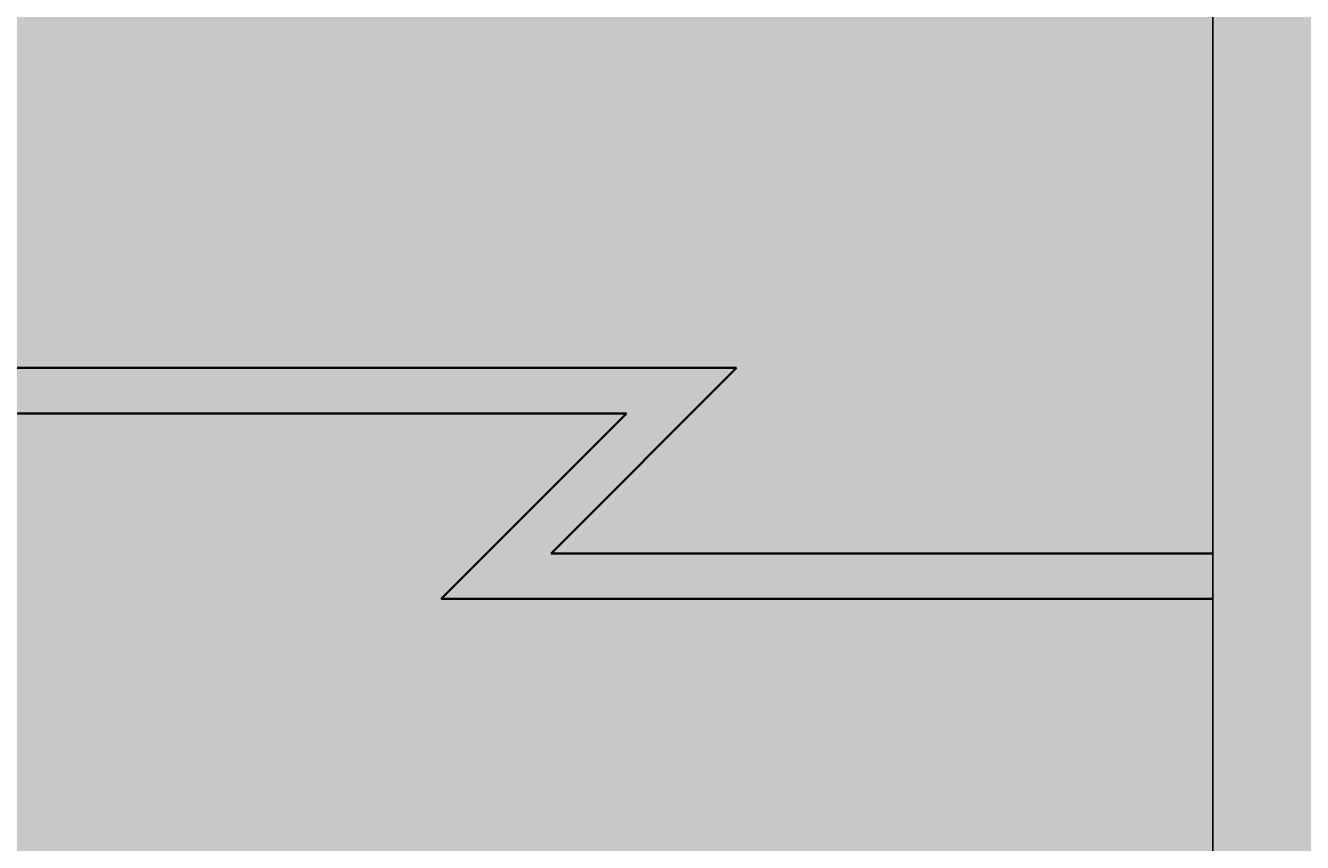
# Model space of a CAD drawing. Units: millimetres. Extents: x -22994 to 29398, y -19990 to 20176.
# Tile 47 of 135: x 170 to 198, y 78 to 96. Entities that reach past the tile are written whole.
import ezdxf
from ezdxf import colors
from ezdxf.entities.mleader import LeaderData, LeaderLine
from ezdxf.math import Vec2, Vec3

# ---------------------------------------------------------------- set-up
doc = ezdxf.new("R2010")
doc.units = ezdxf.units.MM
doc.header["$MEASUREMENT"] = 0
for name, color, linetype, lineweight in [('M-ANNO-TEXT', 7, 'Continuous', 25), ('M-DIMS', 2, 'Continuous', 18), ('M-EQPM', 7, 'Continuous', 25), ('M-EQPM-PATT', 7, 'Continuous', 18), ('M-PIPE', 7, 'Continuous', 35)]:
    doc.layers.add(name, color=color, linetype=linetype, lineweight=lineweight)
doc.styles.get("Standard").update_dxf_attribs({"font": 'arial.ttf'})
doc.dimstyles.get("Standard").update_dxf_attribs({"dimtxt": 0.18, "dimasz": 10000, "dimexe": 0.18, "dimexo": 0.0625, "dimgap": 0.09, "dimtad": 0, "dimtih": 1, "dimtoh": 1, "dimdec": 0, "dimzin": 0, "dimdsep": 46, "dimtxsty": 'Standard', "dimcen": 0.09, "dimadec": 0, "dimazin": 0, "dimtfac": 1, "dimtdec": 0, "dimtofl": 0, "dimtmove": 0, "dimatfit": 3, "dimfxl": 1, "dimtolj": 1, "dimtzin": 0, "dimlwd": 30, "dimarcsym": 0})

# ---------------------------------------------------------------- blocks, each defined once
blk = doc.blocks.new('*D2')
at = {"layer": 'Defpoints', "color": 0, "transparency": 16777216}
for p in [(6.677, 10.271), (290.852, 10.271), (290.852, -5.079)]:
    blk.add_point(p, dxfattribs=at)
at = {"layer": 'M-DIMS', "color": 0, "lineweight": -2, "transparency": 16777216}
for p, q in [((6.677, 10.209), (6.677, -5.259)), ((290.852, 10.209), (290.852, -5.259))]:
    blk.add_line(p, q, dxfattribs=at)
at = {"layer": 'M-DIMS', "color": 0, "lineweight": 30, "transparency": 16777216}
for p, q in [((-9993.323, -5.079), (-19993.323, -5.079)), ((10290.852, -5.079), (20290.852, -5.079))]:
    blk.add_line(p, q, dxfattribs=at)
at = {"layer": 'M-DIMS', "color": 0, "transparency": 16777216}
for points in [[(-9993.323, 1661.588), (-9993.323, -1671.745), (6.677, -5.079)], [(10290.852, 1661.588), (10290.852, -1671.745), (290.852, -5.079)]]:
    blk.add_solid(points, dxfattribs=at)
at = {"layer": 'M-DIMS', "color": 0, "transparency": 16777216, "insert": (148.765, -5.079), "char_height": 0.18, "attachment_point": 5}
blk.add_mtext('\\A1;284.2', dxfattribs=at)
blk = doc.blocks.new('*D3')
at = {"layer": 'Defpoints', "color": 0, "transparency": 16777216}
for p in [(110.265, 204.165), (110.265, 176.366), (95.833, 127.967)]:
    blk.add_point(p, dxfattribs=at)
at = {"layer": 'M-DIMS', "color": 0, "lineweight": 30, "transparency": 16777216}
for p, q in [((-9904.167, 204.165), (-19904.167, 204.165)), ((10110.265, 204.165), (20110.265, 204.165))]:
    blk.add_line(p, q, dxfattribs=at)
at = {"layer": 'M-DIMS', "color": 0, "lineweight": -2, "transparency": 16777216}
for p, q in [((95.833, 128.03), (95.833, 204.345)), ((110.265, 176.429), (110.265, 204.345))]:
    blk.add_line(p, q, dxfattribs=at)
at = {"layer": 'M-DIMS', "color": 0, "transparency": 16777216}
for points in [[(-9904.167, 1870.832), (-9904.167, -1462.501), (95.833, 204.165)], [(10110.265, 1870.832), (10110.265, -1462.501), (110.265, 204.165)]]:
    blk.add_solid(points, dxfattribs=at)
at = {"layer": 'M-DIMS', "color": 0, "transparency": 16777216, "insert": (103.049, 204.165), "char_height": 0.18, "attachment_point": 5}
blk.add_mtext('\\A1;14.432', dxfattribs=at)
blk = doc.blocks.new('*D4')
at = {"layer": 'Defpoints', "color": 0, "transparency": 16777216}
for p in [(116.265, 204.165), (110.265, 176.366), (116.265, 176.366)]:
    blk.add_point(p, dxfattribs=at)
at = {"layer": 'M-DIMS', "color": 0, "lineweight": 30, "transparency": 16777216}
for p, q in [((-9889.735, 204.165), (-19889.735, 204.165)), ((10116.265, 204.165), (20116.265, 204.165))]:
    blk.add_line(p, q, dxfattribs=at)
at = {"layer": 'M-DIMS', "color": 0, "lineweight": -2, "transparency": 16777216}
for p, q in [((110.265, 176.429), (110.265, 204.345)), ((116.265, 176.429), (116.265, 204.345))]:
    blk.add_line(p, q, dxfattribs=at)
at = {"layer": 'M-DIMS', "color": 0, "transparency": 16777216}
for points in [[(-9889.735, 1870.832), (-9889.735, -1462.501), (110.265, 204.165)], [(10116.265, 1870.832), (10116.265, -1462.501), (116.265, 204.165)]]:
    blk.add_solid(points, dxfattribs=at)
at = {"layer": 'M-DIMS', "color": 0, "transparency": 16777216, "insert": (113.265, 204.165), "char_height": 0.18, "attachment_point": 5}
blk.add_mtext('\\A1;6', dxfattribs=at)
blk = doc.blocks.new('*D5')
at = {"layer": 'Defpoints', "color": 0, "transparency": 16777216}
for p in [(181.265, 204.165), (116.265, 176.366), (181.265, 176.366)]:
    blk.add_point(p, dxfattribs=at)
at = {"layer": 'M-DIMS', "color": 0, "lineweight": 30, "transparency": 16777216}
for p, q in [((-9883.735, 204.165), (-19883.735, 204.165)), ((10181.265, 204.165), (20181.265, 204.165))]:
    blk.add_line(p, q, dxfattribs=at)
at = {"layer": 'M-DIMS', "color": 0, "lineweight": -2, "transparency": 16777216}
for p, q in [((116.265, 176.429), (116.265, 204.345)), ((181.265, 176.429), (181.265, 204.345))]:
    blk.add_line(p, q, dxfattribs=at)
at = {"layer": 'M-DIMS', "color": 0, "transparency": 16777216}
for points in [[(-9883.735, 1870.832), (-9883.735, -1462.501), (116.265, 204.165)], [(10181.265, 1870.832), (10181.265, -1462.501), (181.265, 204.165)]]:
    blk.add_solid(points, dxfattribs=at)
at = {"layer": 'M-DIMS', "color": 0, "transparency": 16777216, "insert": (148.765, 204.165), "char_height": 0.18, "attachment_point": 5}
blk.add_mtext('\\A1;65', dxfattribs=at)
blk = doc.blocks.new('*D6')
at = {"layer": 'Defpoints', "color": 0, "transparency": 16777216}
for p in [(187.265, 204.165), (181.265, 176.366), (187.265, 176.366)]:
    blk.add_point(p, dxfattribs=at)
at = {"layer": 'M-DIMS', "color": 0, "lineweight": 30, "transparency": 16777216}
for p, q in [((-9818.735, 204.165), (-19818.735, 204.165)), ((10187.265, 204.165), (20187.265, 204.165))]:
    blk.add_line(p, q, dxfattribs=at)
at = {"layer": 'M-DIMS', "color": 0, "lineweight": -2, "transparency": 16777216}
for p, q in [((181.265, 176.429), (181.265, 204.345)), ((187.265, 176.429), (187.265, 204.345))]:
    blk.add_line(p, q, dxfattribs=at)
at = {"layer": 'M-DIMS', "color": 0, "transparency": 16777216}
for points in [[(-9818.735, 1870.832), (-9818.735, -1462.501), (181.265, 204.165)], [(10187.265, 1870.832), (10187.265, -1462.501), (187.265, 204.165)]]:
    blk.add_solid(points, dxfattribs=at)
at = {"layer": 'M-DIMS', "color": 0, "transparency": 16777216, "insert": (184.265, 204.165), "char_height": 0.18, "attachment_point": 5}
blk.add_mtext('\\A1;6', dxfattribs=at)
blk = doc.blocks.new('*D7')
at = {"layer": 'Defpoints', "color": 0, "transparency": 16777216}
for p in [(201.697, 204.165), (187.265, 176.366), (201.697, 127.967)]:
    blk.add_point(p, dxfattribs=at)
at = {"layer": 'M-DIMS', "color": 0, "lineweight": 30, "transparency": 16777216}
for p, q in [((-9812.735, 204.165), (-19812.735, 204.165)), ((10201.697, 204.165), (20201.697, 204.165))]:
    blk.add_line(p, q, dxfattribs=at)
at = {"layer": 'M-DIMS', "color": 0, "lineweight": -2, "transparency": 16777216}
for p, q in [((187.265, 176.429), (187.265, 204.345)), ((201.697, 128.03), (201.697, 204.345))]:
    blk.add_line(p, q, dxfattribs=at)
at = {"layer": 'M-DIMS', "color": 0, "transparency": 16777216}
for points in [[(-9812.735, 1870.832), (-9812.735, -1462.501), (187.265, 204.165)], [(10201.697, 1870.832), (10201.697, -1462.501), (201.697, 204.165)]]:
    blk.add_solid(points, dxfattribs=at)
at = {"layer": 'M-DIMS', "color": 0, "transparency": 16777216, "insert": (194.481, 204.165), "char_height": 0.18, "attachment_point": 5}
blk.add_mtext('\\A1;14.432', dxfattribs=at)
blk = doc.blocks.new('*D8')
at = {"layer": 'Defpoints', "color": 0, "transparency": 16777216}
for p in [(227.648, 204.165), (227.648, 146.73), (201.697, 127.967)]:
    blk.add_point(p, dxfattribs=at)
at = {"layer": 'M-DIMS', "color": 0, "lineweight": 30, "transparency": 16777216}
for p, q in [((-9798.303, 204.165), (-19798.303, 204.165)), ((10227.648, 204.165), (20227.648, 204.165))]:
    blk.add_line(p, q, dxfattribs=at)
at = {"layer": 'M-DIMS', "color": 0, "lineweight": -2, "transparency": 16777216}
for p, q in [((201.697, 128.03), (201.697, 204.345)), ((227.648, 146.792), (227.648, 204.345))]:
    blk.add_line(p, q, dxfattribs=at)
at = {"layer": 'M-DIMS', "color": 0, "transparency": 16777216}
for points in [[(-9798.303, 1870.832), (-9798.303, -1462.501), (201.697, 204.165)], [(10227.648, 1870.832), (10227.648, -1462.501), (227.648, 204.165)]]:
    blk.add_solid(points, dxfattribs=at)
at = {"layer": 'M-DIMS', "color": 0, "transparency": 16777216, "insert": (214.673, 204.165), "char_height": 0.18, "attachment_point": 5}
blk.add_mtext('\\A1;25.95', dxfattribs=at)
blk = doc.blocks.new('*D9')
at = {"layer": 'Defpoints', "color": 0, "transparency": 16777216}
for p in [(187.265, 176.366), (306.202, 176.366), (290.852, 10.271)]:
    blk.add_point(p, dxfattribs=at)
at = {"layer": 'M-DIMS', "color": 0, "lineweight": 30, "transparency": 16777216}
for p, q in [((306.202, 10176.366), (306.202, 20176.366)), ((306.202, -9989.729), (306.202, -19989.729))]:
    blk.add_line(p, q, dxfattribs=at)
at = {"layer": 'M-DIMS', "color": 0, "lineweight": -2, "transparency": 16777216}
for p, q in [((187.327, 176.366), (306.382, 176.366)), ((290.915, 10.271), (306.382, 10.271))]:
    blk.add_line(p, q, dxfattribs=at)
at = {"layer": 'M-DIMS', "color": 0, "transparency": 16777216}
for points in [[(-1360.465, 10176.366), (1972.869, 10176.366), (306.202, 176.366)], [(-1360.465, -9989.729), (1972.869, -9989.729), (306.202, 10.271)]]:
    blk.add_solid(points, dxfattribs=at)
at = {"layer": 'M-DIMS', "color": 0, "transparency": 16777216, "insert": (306.202, 93.319), "char_height": 0.18, "attachment_point": 5}
blk.add_mtext('\\A1;166.1', dxfattribs=at)
blk = doc.blocks.new('*D10')
at = {"layer": 'Defpoints', "color": 0, "transparency": 16777216}
for p in [(125.65, 136.071), (133.346, 136.071), (133.346, -5.079)]:
    blk.add_point(p, dxfattribs=at)
at = {"layer": 'M-DIMS', "color": 0, "lineweight": -2, "transparency": 16777216}
for p, q in [((125.65, 136.009), (125.65, -5.259)), ((133.346, 136.009), (133.346, -5.259))]:
    blk.add_line(p, q, dxfattribs=at)
at = {"layer": 'M-DIMS', "color": 0, "lineweight": 30, "transparency": 16777216}
for p, q in [((-9874.35, -5.079), (-19874.35, -5.079)), ((10133.346, -5.079), (20133.346, -5.079))]:
    blk.add_line(p, q, dxfattribs=at)
at = {"layer": 'M-DIMS', "color": 0, "transparency": 16777216}
for points in [[(-9874.35, 1661.588), (-9874.35, -1671.745), (125.65, -5.079)], [(10133.346, 1661.588), (10133.346, -1671.745), (133.346, -5.079)]]:
    blk.add_solid(points, dxfattribs=at)
at = {"layer": 'M-DIMS', "color": 0, "transparency": 16777216, "insert": (129.498, -5.079), "char_height": 0.18, "attachment_point": 5}
blk.add_mtext('\\A1;7.696', dxfattribs=at)
blk = doc.blocks.new('*D11')
at = {"layer": 'Defpoints', "color": 0, "transparency": 16777216}
for p in [(133.346, 136.071), (135.65, 136.071), (135.65, -5.079)]:
    blk.add_point(p, dxfattribs=at)
at = {"layer": 'M-DIMS', "color": 0, "lineweight": -2, "transparency": 16777216}
for p, q in [((133.346, 136.009), (133.346, -5.259)), ((135.65, 136.009), (135.65, -5.259))]:
    blk.add_line(p, q, dxfattribs=at)
at = {"layer": 'M-DIMS', "color": 0, "lineweight": 30, "transparency": 16777216}
for p, q in [((-9866.654, -5.079), (-19866.654, -5.079)), ((10135.65, -5.079), (20135.65, -5.079))]:
    blk.add_line(p, q, dxfattribs=at)
at = {"layer": 'M-DIMS', "color": 0, "transparency": 16777216}
for points in [[(-9866.654, 1661.588), (-9866.654, -1671.745), (133.346, -5.079)], [(10135.65, 1661.588), (10135.65, -1671.745), (135.65, -5.079)]]:
    blk.add_solid(points, dxfattribs=at)
at = {"layer": 'M-DIMS', "color": 0, "transparency": 16777216, "insert": (134.498, -5.079), "char_height": 0.18, "attachment_point": 5}
blk.add_mtext('\\A1;2.304', dxfattribs=at)
blk = doc.blocks.new('*D12')
at = {"layer": 'Defpoints', "color": 0, "transparency": 16777216}
for p in [(135.65, 136.071), (145.65, 136.071), (145.65, -5.079)]:
    blk.add_point(p, dxfattribs=at)
at = {"layer": 'M-DIMS', "color": 0, "lineweight": -2, "transparency": 16777216}
for p, q in [((135.65, 136.009), (135.65, -5.259)), ((145.65, 136.009), (145.65, -5.259))]:
    blk.add_line(p, q, dxfattribs=at)
at = {"layer": 'M-DIMS', "color": 0, "lineweight": 30, "transparency": 16777216}
for p, q in [((-9864.35, -5.079), (-19864.35, -5.079)), ((10145.65, -5.079), (20145.65, -5.079))]:
    blk.add_line(p, q, dxfattribs=at)
at = {"layer": 'M-DIMS', "color": 0, "transparency": 16777216}
for points in [[(-9864.35, 1661.588), (-9864.35, -1671.745), (135.65, -5.079)], [(10145.65, 1661.588), (10145.65, -1671.745), (145.65, -5.079)]]:
    blk.add_solid(points, dxfattribs=at)
at = {"layer": 'M-DIMS', "color": 0, "transparency": 16777216, "insert": (140.65, -5.079), "char_height": 0.18, "attachment_point": 5}
blk.add_mtext('\\A1;10', dxfattribs=at)
blk = doc.blocks.new('*D13')
at = {"layer": 'Defpoints', "color": 0, "transparency": 16777216}
for p in [(145.65, 136.071), (155.65, 136.071), (155.65, -5.079)]:
    blk.add_point(p, dxfattribs=at)
at = {"layer": 'M-DIMS', "color": 0, "lineweight": -2, "transparency": 16777216}
for p, q in [((145.65, 136.009), (145.65, -5.259)), ((155.65, 136.009), (155.65, -5.259))]:
    blk.add_line(p, q, dxfattribs=at)
at = {"layer": 'M-DIMS', "color": 0, "lineweight": 30, "transparency": 16777216}
for p, q in [((-9854.35, -5.079), (-19854.35, -5.079)), ((10155.65, -5.079), (20155.65, -5.079))]:
    blk.add_line(p, q, dxfattribs=at)
at = {"layer": 'M-DIMS', "color": 0, "transparency": 16777216}
for points in [[(-9854.35, 1661.588), (-9854.35, -1671.745), (145.65, -5.079)], [(10155.65, 1661.588), (10155.65, -1671.745), (155.65, -5.079)]]:
    blk.add_solid(points, dxfattribs=at)
at = {"layer": 'M-DIMS', "color": 0, "transparency": 16777216, "insert": (150.65, -5.079), "char_height": 0.18, "attachment_point": 5}
blk.add_mtext('\\A1;10', dxfattribs=at)
blk = doc.blocks.new('*D14')
at = {"layer": 'Defpoints', "color": 0, "transparency": 16777216}
for p in [(155.65, 136.071), (165.65, 136.071), (165.65, -5.079)]:
    blk.add_point(p, dxfattribs=at)
at = {"layer": 'M-DIMS', "color": 0, "lineweight": -2, "transparency": 16777216}
for p, q in [((155.65, 136.009), (155.65, -5.259)), ((165.65, 136.009), (165.65, -5.259))]:
    blk.add_line(p, q, dxfattribs=at)
at = {"layer": 'M-DIMS', "color": 0, "lineweight": 30, "transparency": 16777216}
for p, q in [((-9844.35, -5.079), (-19844.35, -5.079)), ((10165.65, -5.079), (20165.65, -5.079))]:
    blk.add_line(p, q, dxfattribs=at)
at = {"layer": 'M-DIMS', "color": 0, "transparency": 16777216}
for points in [[(-9844.35, 1661.588), (-9844.35, -1671.745), (155.65, -5.079)], [(10165.65, 1661.588), (10165.65, -1671.745), (165.65, -5.079)]]:
    blk.add_solid(points, dxfattribs=at)
at = {"layer": 'M-DIMS', "color": 0, "transparency": 16777216, "insert": (160.65, -5.079), "char_height": 0.18, "attachment_point": 5}
blk.add_mtext('\\A1;10', dxfattribs=at)
blk = doc.blocks.new('*D15')
at = {"layer": 'Defpoints', "color": 0, "transparency": 16777216}
for p in [(173.346, 154.788), (173.346, 136.071), (306.202, 136.071)]:
    blk.add_point(p, dxfattribs=at)
at = {"layer": 'M-DIMS', "color": 0, "lineweight": 30, "transparency": 16777216}
for p, q in [((306.202, 10154.788), (306.202, 20154.788)), ((306.202, -9863.929), (306.202, -19863.929))]:
    blk.add_line(p, q, dxfattribs=at)
at = {"layer": 'M-DIMS', "color": 0, "lineweight": -2, "transparency": 16777216}
for p, q in [((173.408, 154.788), (306.382, 154.788)), ((173.408, 136.071), (306.382, 136.071))]:
    blk.add_line(p, q, dxfattribs=at)
at = {"layer": 'M-DIMS', "color": 0, "transparency": 16777216}
for points in [[(-1360.465, 10154.788), (1972.869, 10154.788), (306.202, 154.788)], [(-1360.465, -9863.929), (1972.869, -9863.929), (306.202, 136.071)]]:
    blk.add_solid(points, dxfattribs=at)
at = {"layer": 'M-DIMS', "color": 0, "transparency": 16777216, "insert": (306.202, 145.43), "char_height": 0.18, "attachment_point": 5}
blk.add_mtext('\\A1;18.717', dxfattribs=at)
blk = doc.blocks.new('*D16')
at = {"layer": 'Defpoints', "color": 0, "transparency": 16777216}
for p in [(120.17, 204.165), (110.466, 48.035), (120.17, 48.035)]:
    blk.add_point(p, dxfattribs=at)
at = {"layer": 'M-DIMS', "color": 0, "lineweight": 30, "transparency": 16777216}
for p, q in [((-9889.534, 204.165), (-19889.534, 204.165)), ((10120.17, 204.165), (20120.17, 204.165))]:
    blk.add_line(p, q, dxfattribs=at)
at = {"layer": 'M-DIMS', "color": 0, "lineweight": -2, "transparency": 16777216}
for p, q in [((110.466, 48.097), (110.466, 204.345)), ((120.17, 48.097), (120.17, 204.345))]:
    blk.add_line(p, q, dxfattribs=at)
at = {"layer": 'M-DIMS', "color": 0, "transparency": 16777216}
for points in [[(-9889.534, 1870.832), (-9889.534, -1462.501), (110.466, 204.165)], [(10120.17, 1870.832), (10120.17, -1462.501), (120.17, 204.165)]]:
    blk.add_solid(points, dxfattribs=at)
at = {"layer": 'M-DIMS', "color": 0, "transparency": 16777216, "insert": (115.318, 204.165), "char_height": 0.18, "attachment_point": 5}
blk.add_mtext('\\A1;9.704', dxfattribs=at)
blk = doc.blocks.new('*D17')
at = {"layer": 'Defpoints', "color": 0, "transparency": 16777216}
for p in [(126.17, 204.165), (120.17, 48.035), (126.17, 48.035)]:
    blk.add_point(p, dxfattribs=at)
at = {"layer": 'M-DIMS', "color": 0, "lineweight": 30, "transparency": 16777216}
for p, q in [((-9879.83, 204.165), (-19879.83, 204.165)), ((10126.17, 204.165), (20126.17, 204.165))]:
    blk.add_line(p, q, dxfattribs=at)
at = {"layer": 'M-DIMS', "color": 0, "lineweight": -2, "transparency": 16777216}
for p, q in [((120.17, 48.097), (120.17, 204.345)), ((126.17, 48.097), (126.17, 204.345))]:
    blk.add_line(p, q, dxfattribs=at)
at = {"layer": 'M-DIMS', "color": 0, "transparency": 16777216}
for points in [[(-9879.83, 1870.832), (-9879.83, -1462.501), (120.17, 204.165)], [(10126.17, 1870.832), (10126.17, -1462.501), (126.17, 204.165)]]:
    blk.add_solid(points, dxfattribs=at)
at = {"layer": 'M-DIMS', "color": 0, "transparency": 16777216, "insert": (123.17, 204.165), "char_height": 0.18, "attachment_point": 5}
blk.add_mtext('\\A1;6', dxfattribs=at)
blk = doc.blocks.new('*D18')
at = {"layer": 'Defpoints', "color": 0, "transparency": 16777216}
for p in [(132.17, 204.165), (126.17, 48.035), (132.17, 48.035)]:
    blk.add_point(p, dxfattribs=at)
at = {"layer": 'M-DIMS', "color": 0, "lineweight": 30, "transparency": 16777216}
for p, q in [((-9873.83, 204.165), (-19873.83, 204.165)), ((10132.17, 204.165), (20132.17, 204.165))]:
    blk.add_line(p, q, dxfattribs=at)
at = {"layer": 'M-DIMS', "color": 0, "lineweight": -2, "transparency": 16777216}
for p, q in [((126.17, 48.097), (126.17, 204.345)), ((132.17, 48.097), (132.17, 204.345))]:
    blk.add_line(p, q, dxfattribs=at)
at = {"layer": 'M-DIMS', "color": 0, "transparency": 16777216}
for points in [[(-9873.83, 1870.832), (-9873.83, -1462.501), (126.17, 204.165)], [(10132.17, 1870.832), (10132.17, -1462.501), (132.17, 204.165)]]:
    blk.add_solid(points, dxfattribs=at)
at = {"layer": 'M-DIMS', "color": 0, "transparency": 16777216, "insert": (129.17, 204.165), "char_height": 0.18, "attachment_point": 5}
blk.add_mtext('\\A1;6', dxfattribs=at)
blk = doc.blocks.new('*D19')
at = {"layer": 'Defpoints', "color": 0, "transparency": 16777216}
for p in [(138.17, 204.165), (132.17, 48.035), (138.17, 48.035)]:
    blk.add_point(p, dxfattribs=at)
at = {"layer": 'M-DIMS', "color": 0, "lineweight": 30, "transparency": 16777216}
for p, q in [((-9867.83, 204.165), (-19867.83, 204.165)), ((10138.17, 204.165), (20138.17, 204.165))]:
    blk.add_line(p, q, dxfattribs=at)
at = {"layer": 'M-DIMS', "color": 0, "lineweight": -2, "transparency": 16777216}
for p, q in [((132.17, 48.097), (132.17, 204.345)), ((138.17, 48.097), (138.17, 204.345))]:
    blk.add_line(p, q, dxfattribs=at)
at = {"layer": 'M-DIMS', "color": 0, "transparency": 16777216}
for points in [[(-9867.83, 1870.832), (-9867.83, -1462.501), (132.17, 204.165)], [(10138.17, 1870.832), (10138.17, -1462.501), (138.17, 204.165)]]:
    blk.add_solid(points, dxfattribs=at)
at = {"layer": 'M-DIMS', "color": 0, "transparency": 16777216, "insert": (135.17, 204.165), "char_height": 0.18, "attachment_point": 5}
blk.add_mtext('\\A1;6', dxfattribs=at)
blk = doc.blocks.new('*D20')
at = {"layer": 'Defpoints', "color": 0, "transparency": 16777216}
for p in [(144.17, 204.165), (138.17, 48.035), (144.17, 48.035)]:
    blk.add_point(p, dxfattribs=at)
at = {"layer": 'M-DIMS', "color": 0, "lineweight": 30, "transparency": 16777216}
for p, q in [((-9861.83, 204.165), (-19861.83, 204.165)), ((10144.17, 204.165), (20144.17, 204.165))]:
    blk.add_line(p, q, dxfattribs=at)
at = {"layer": 'M-DIMS', "color": 0, "lineweight": -2, "transparency": 16777216}
for p, q in [((138.17, 48.097), (138.17, 204.345)), ((144.17, 48.097), (144.17, 204.345))]:
    blk.add_line(p, q, dxfattribs=at)
at = {"layer": 'M-DIMS', "color": 0, "transparency": 16777216}
for points in [[(-9861.83, 1870.832), (-9861.83, -1462.501), (138.17, 204.165)], [(10144.17, 1870.832), (10144.17, -1462.501), (144.17, 204.165)]]:
    blk.add_solid(points, dxfattribs=at)
at = {"layer": 'M-DIMS', "color": 0, "transparency": 16777216, "insert": (141.17, 204.165), "char_height": 0.18, "attachment_point": 5}
blk.add_mtext('\\A1;6', dxfattribs=at)
blk = doc.blocks.new('*D21')
at = {"layer": 'Defpoints', "color": 0, "transparency": 16777216}
for p in [(149.116, 204.165), (144.17, 48.035), (149.116, 48.035)]:
    blk.add_point(p, dxfattribs=at)
at = {"layer": 'M-DIMS', "color": 0, "lineweight": 30, "transparency": 16777216}
for p, q in [((-9855.83, 204.165), (-19855.83, 204.165)), ((10149.116, 204.165), (20149.116, 204.165))]:
    blk.add_line(p, q, dxfattribs=at)
at = {"layer": 'M-DIMS', "color": 0, "lineweight": -2, "transparency": 16777216}
for p, q in [((144.17, 48.097), (144.17, 204.345)), ((149.116, 48.097), (149.116, 204.345))]:
    blk.add_line(p, q, dxfattribs=at)
at = {"layer": 'M-DIMS', "color": 0, "transparency": 16777216}
for points in [[(-9855.83, 1870.832), (-9855.83, -1462.501), (144.17, 204.165)], [(10149.116, 1870.832), (10149.116, -1462.501), (149.116, 204.165)]]:
    blk.add_solid(points, dxfattribs=at)
at = {"layer": 'M-DIMS', "color": 0, "transparency": 16777216, "insert": (146.643, 204.165), "char_height": 0.18, "attachment_point": 5}
blk.add_mtext('\\A1;4.945', dxfattribs=at)
blk = doc.blocks.new('*D22')
at = {"layer": 'Defpoints', "color": 0, "transparency": 16777216}
for p in [(149.116, 30.99), (155.116, 30.99), (155.116, -5.079)]:
    blk.add_point(p, dxfattribs=at)
at = {"layer": 'M-DIMS', "color": 0, "lineweight": -2, "transparency": 16777216}
for p, q in [((149.116, 30.927), (149.116, -5.259)), ((155.116, 30.927), (155.116, -5.259))]:
    blk.add_line(p, q, dxfattribs=at)
at = {"layer": 'M-DIMS', "color": 0, "lineweight": 30, "transparency": 16777216}
for p, q in [((-9850.884, -5.079), (-19850.884, -5.079)), ((10155.116, -5.079), (20155.116, -5.079))]:
    blk.add_line(p, q, dxfattribs=at)
at = {"layer": 'M-DIMS', "color": 0, "transparency": 16777216}
for points in [[(-9850.884, 1661.588), (-9850.884, -1671.745), (149.116, -5.079)], [(10155.116, 1661.588), (10155.116, -1671.745), (155.116, -5.079)]]:
    blk.add_solid(points, dxfattribs=at)
at = {"layer": 'M-DIMS', "color": 0, "transparency": 16777216, "insert": (152.116, -5.079), "char_height": 0.18, "attachment_point": 5}
blk.add_mtext('\\A1;6', dxfattribs=at)
blk = doc.blocks.new('*D23')
at = {"layer": 'Defpoints', "color": 0, "transparency": 16777216}
for p in [(155.116, 30.99), (161.116, 30.99), (161.116, -5.079)]:
    blk.add_point(p, dxfattribs=at)
at = {"layer": 'M-DIMS', "color": 0, "lineweight": -2, "transparency": 16777216}
for p, q in [((155.116, 30.927), (155.116, -5.259)), ((161.116, 30.927), (161.116, -5.259))]:
    blk.add_line(p, q, dxfattribs=at)
at = {"layer": 'M-DIMS', "color": 0, "lineweight": 30, "transparency": 16777216}
for p, q in [((-9844.884, -5.079), (-19844.884, -5.079)), ((10161.116, -5.079), (20161.116, -5.079))]:
    blk.add_line(p, q, dxfattribs=at)
at = {"layer": 'M-DIMS', "color": 0, "transparency": 16777216}
for points in [[(-9844.884, 1661.588), (-9844.884, -1671.745), (155.116, -5.079)], [(10161.116, 1661.588), (10161.116, -1671.745), (161.116, -5.079)]]:
    blk.add_solid(points, dxfattribs=at)
at = {"layer": 'M-DIMS', "color": 0, "transparency": 16777216, "insert": (158.116, -5.079), "char_height": 0.18, "attachment_point": 5}
blk.add_mtext('\\A1;6', dxfattribs=at)
blk = doc.blocks.new('*D24')
at = {"layer": 'Defpoints', "color": 0, "transparency": 16777216}
for p in [(161.116, 30.99), (166.439, 30.99), (166.439, -5.079)]:
    blk.add_point(p, dxfattribs=at)
at = {"layer": 'M-DIMS', "color": 0, "lineweight": -2, "transparency": 16777216}
for p, q in [((161.116, 30.927), (161.116, -5.259)), ((166.439, 30.927), (166.439, -5.259))]:
    blk.add_line(p, q, dxfattribs=at)
at = {"layer": 'M-DIMS', "color": 0, "lineweight": 30, "transparency": 16777216}
for p, q in [((-9838.884, -5.079), (-19838.884, -5.079)), ((10166.439, -5.079), (20166.439, -5.079))]:
    blk.add_line(p, q, dxfattribs=at)
at = {"layer": 'M-DIMS', "color": 0, "transparency": 16777216}
for points in [[(-9838.884, 1661.588), (-9838.884, -1671.745), (161.116, -5.079)], [(10166.439, 1661.588), (10166.439, -1671.745), (166.439, -5.079)]]:
    blk.add_solid(points, dxfattribs=at)
at = {"layer": 'M-DIMS', "color": 0, "transparency": 16777216, "insert": (163.777, -5.079), "char_height": 0.18, "attachment_point": 5}
blk.add_mtext('\\A1;5.323', dxfattribs=at)
blk = doc.blocks.new('*D25')
at = {"layer": 'Defpoints', "color": 0, "transparency": 16777216}
for p in [(166.439, 30.99), (172.439, 30.99), (172.439, -5.079)]:
    blk.add_point(p, dxfattribs=at)
at = {"layer": 'M-DIMS', "color": 0, "lineweight": -2, "transparency": 16777216}
for p, q in [((166.439, 30.927), (166.439, -5.259)), ((172.439, 30.927), (172.439, -5.259))]:
    blk.add_line(p, q, dxfattribs=at)
at = {"layer": 'M-DIMS', "color": 0, "lineweight": 30, "transparency": 16777216}
for p, q in [((-9833.561, -5.079), (-19833.561, -5.079)), ((10172.439, -5.079), (20172.439, -5.079))]:
    blk.add_line(p, q, dxfattribs=at)
at = {"layer": 'M-DIMS', "color": 0, "transparency": 16777216}
for points in [[(-9833.561, 1661.588), (-9833.561, -1671.745), (166.439, -5.079)], [(10172.439, 1661.588), (10172.439, -1671.745), (172.439, -5.079)]]:
    blk.add_solid(points, dxfattribs=at)
at = {"layer": 'M-DIMS', "color": 0, "transparency": 16777216, "insert": (169.439, -5.079), "char_height": 0.18, "attachment_point": 5}
blk.add_mtext('\\A1;6', dxfattribs=at)
blk = doc.blocks.new('*D26')
at = {"layer": 'Defpoints', "color": 0, "transparency": 16777216}
for p in [(172.439, 30.99), (178.439, 30.99), (178.439, -5.079)]:
    blk.add_point(p, dxfattribs=at)
at = {"layer": 'M-DIMS', "color": 0, "lineweight": -2, "transparency": 16777216}
for p, q in [((172.439, 30.927), (172.439, -5.259)), ((178.439, 30.927), (178.439, -5.259))]:
    blk.add_line(p, q, dxfattribs=at)
at = {"layer": 'M-DIMS', "color": 0, "lineweight": 30, "transparency": 16777216}
for p, q in [((-9827.561, -5.079), (-19827.561, -5.079)), ((10178.439, -5.079), (20178.439, -5.079))]:
    blk.add_line(p, q, dxfattribs=at)
at = {"layer": 'M-DIMS', "color": 0, "transparency": 16777216}
for points in [[(-9827.561, 1661.588), (-9827.561, -1671.745), (172.439, -5.079)], [(10178.439, 1661.588), (10178.439, -1671.745), (178.439, -5.079)]]:
    blk.add_solid(points, dxfattribs=at)
at = {"layer": 'M-DIMS', "color": 0, "transparency": 16777216, "insert": (175.439, -5.079), "char_height": 0.18, "attachment_point": 5}
blk.add_mtext('\\A1;6', dxfattribs=at)
blk = doc.blocks.new('*D27')
at = {"layer": 'Defpoints', "color": 0, "transparency": 16777216}
for p in [(178.439, 30.99), (188.117, 30.99), (188.117, -5.079)]:
    blk.add_point(p, dxfattribs=at)
at = {"layer": 'M-DIMS', "color": 0, "lineweight": -2, "transparency": 16777216}
for p, q in [((178.439, 30.927), (178.439, -5.259)), ((188.117, 30.927), (188.117, -5.259))]:
    blk.add_line(p, q, dxfattribs=at)
at = {"layer": 'M-DIMS', "color": 0, "lineweight": 30, "transparency": 16777216}
for p, q in [((-9821.561, -5.079), (-19821.561, -5.079)), ((10188.117, -5.079), (20188.117, -5.079))]:
    blk.add_line(p, q, dxfattribs=at)
at = {"layer": 'M-DIMS', "color": 0, "transparency": 16777216}
for points in [[(-9821.561, 1661.588), (-9821.561, -1671.745), (178.439, -5.079)], [(10188.117, 1661.588), (10188.117, -1671.745), (188.117, -5.079)]]:
    blk.add_solid(points, dxfattribs=at)
at = {"layer": 'M-DIMS', "color": 0, "transparency": 16777216, "insert": (183.278, -5.079), "char_height": 0.18, "attachment_point": 5}
blk.add_mtext('\\A1;9.679', dxfattribs=at)
blk = doc.blocks.new('*D28')
at = {"layer": 'Defpoints', "color": 0, "transparency": 16777216}
for p in [(188.117, 48.035), (306.202, 48.035), (188.117, 30.99)]:
    blk.add_point(p, dxfattribs=at)
at = {"layer": 'M-DIMS', "color": 0, "lineweight": 30, "transparency": 16777216}
for p, q in [((306.202, 10048.035), (306.202, 20048.035)), ((306.202, -9969.01), (306.202, -19969.01))]:
    blk.add_line(p, q, dxfattribs=at)
at = {"layer": 'M-DIMS', "color": 0, "lineweight": -2, "transparency": 16777216}
for p, q in [((188.18, 48.035), (306.382, 48.035)), ((188.18, 30.99), (306.382, 30.99))]:
    blk.add_line(p, q, dxfattribs=at)
at = {"layer": 'M-DIMS', "color": 0, "transparency": 16777216}
for points in [[(-1360.465, 10048.035), (1972.869, 10048.035), (306.202, 48.035)], [(-1360.465, -9969.01), (1972.869, -9969.01), (306.202, 30.99)]]:
    blk.add_solid(points, dxfattribs=at)
at = {"layer": 'M-DIMS', "color": 0, "transparency": 16777216, "insert": (306.202, 39.512), "char_height": 0.18, "attachment_point": 5}
blk.add_mtext('\\A1;17.045', dxfattribs=at)
blk = doc.blocks.new('*D29')
at = {"layer": 'Defpoints', "color": 0, "transparency": 16777216}
for p in [(36.801, 80.045), (64.03, 80.045)]:
    blk.add_point(p, dxfattribs=at)
at = {"layer": 'M-DIMS', "color": 0, "lineweight": -2, "transparency": 16777216}
for p, q in [((50.325, 80.045), (50.505, 80.045)), ((50.415, 79.955), (50.415, 80.135))]:
    blk.add_line(p, q, dxfattribs=at)
at = {"layer": 'M-DIMS', "color": 0, "lineweight": 30, "transparency": 16777216}
blk.add_line((20064.03, 80.03), (10064.03, 80.038), dxfattribs=at)
at = {"layer": 'M-DIMS', "color": 0, "transparency": 16777216}
blk.add_solid([(10064.031, 1746.704), (10064.028, -1586.629), (64.03, 80.045)], dxfattribs=at)
at = {"layer": 'M-DIMS', "color": 0, "transparency": 16777216, "insert": (20064.521, 80.03), "char_height": 0.18, "attachment_point": 5}
blk.add_mtext('\\A1;∅27.23', dxfattribs=at)
blk = doc.blocks.new('*D36')
at = {"layer": 'Defpoints', "color": 0, "transparency": 16777216}
for p in [(46.39, 31.303), (46.387, 26.593)]:
    blk.add_point(p, dxfattribs=at)
at = {"layer": 'M-DIMS', "color": 0, "lineweight": 30, "transparency": 16777216}
for p, q in [((57.15, 20031.301), (51.77, 10031.302)), ((10057.15, 20031.301), (57.15, 20031.301))]:
    blk.add_line(p, q, dxfattribs=at)
at = {"layer": 'M-DIMS', "color": 0, "lineweight": -2, "transparency": 16777216}
for p, q in [((46.299, 28.948), (46.479, 28.948)), ((46.389, 28.858), (46.389, 29.038))]:
    blk.add_line(p, q, dxfattribs=at)
at = {"layer": 'M-DIMS', "color": 0, "transparency": 16777216}
blk.add_solid([(-1614.896, 10032.199), (1718.436, 10030.405), (46.39, 31.303)], dxfattribs=at)
at = {"layer": 'M-DIMS', "color": 0, "transparency": 16777216, "insert": (10057.554, 20031.301), "char_height": 0.18, "attachment_point": 5}
blk.add_mtext('\\A1;∅4.71', dxfattribs=at)
blk = doc.blocks.new('*D37')
at = {"layer": 'Defpoints', "color": 0, "transparency": 16777216}
for p in [(54.834, 118.615), (59.494, 118.614)]:
    blk.add_point(p, dxfattribs=at)
at = {"layer": 'M-DIMS', "color": 0, "lineweight": -2, "transparency": 16777216}
for p, q in [((57.074, 118.614), (57.254, 118.614)), ((57.164, 118.524), (57.164, 118.704))]:
    blk.add_line(p, q, dxfattribs=at)
at = {"layer": 'M-DIMS', "color": 0, "lineweight": 30, "transparency": 16777216}
blk.add_line((20059.493, 116.253), (10059.494, 117.434), dxfattribs=at)
at = {"layer": 'M-DIMS', "color": 0, "transparency": 16777216}
blk.add_solid([(10059.69, 1784.1), (10059.297, -1549.233), (59.494, 118.614)], dxfattribs=at)
at = {"layer": 'M-DIMS', "color": 0, "transparency": 16777216, "insert": (20059.985, 116.253), "char_height": 0.18, "attachment_point": 5}
blk.add_mtext('\\A1;∅4.659', dxfattribs=at)

msp = doc.modelspace()

# ---------------------------------------------------------------- hatches: boundary and pattern name
at = {"layer": 'M-EQPM-PATT'}
h = msp.add_hatch(color=256, dxfattribs=at)
h.set_gradient(color1=(205, 32, 39), color2=(205, 32, 39), tint=1)
h.paths.add_polyline_path([(116.2647, 150.3662), (116.2647, 170.3662), (116.2647, 176.3662), (110.2647, 176.3662), (110.2647, 152.0276), (95.8327, 127.967), (95.8327, 16.6063), (201.6967, 16.6063), (201.6967, 127.967), (187.2647, 152.0276), (187.2647, 176.3662), (181.2647, 176.3662), (181.2647, 170.3662), (181.2647, 150.3662), (195.6967, 126.3055), (195.6967, 22.6063), (101.8327, 22.6063), (101.8327, 126.3055)])
h.paths.add_polyline_path([(185.2208, 88.6347), (101.8327, 88.6347), (101.8327, 87.6347), (182.8066, 87.6347), (178.7313, 83.5594), (195.6967, 83.5594), (195.6967, 84.5594), (181.1455, 84.5594)], flags=17)
h.paths.add_polyline_path([(95.8327, 88.6347), (60.9779, 88.6347, -0.0228552), (61.7178, 87.6347), (95.8327, 87.6347)])
h.paths.add_polyline_path([(215.6212, 86.5189), (215.6212, 80.5999), (220.5095, 83.5594)])
h.paths.add_polyline_path([(215.6212, 84.5594), (201.6967, 84.5594), (201.6967, 83.5594), (215.6212, 83.5594)])
h.paths.add_polyline_path([(225.3978, 86.5189), (220.5095, 83.5594), (225.3978, 80.5999)])
h.paths.add_polyline_path([(231.6256, 84.5594), (225.3978, 84.5594), (225.3978, 83.5594), (231.6256, 83.5594)])

# ---------------------------------------------------------------- linework, layer by layer
at = {"layer": 'M-EQPM'}
msp.add_lwpolyline([(116.2647, 170.3662), (116.2647, 150.3662), (101.8327, 126.3055), (101.8327, 22.6063), (195.6967, 22.6063), (195.6967, 126.3055), (181.2647, 150.3662), (181.2647, 170.3662)], dxfattribs=at)
at = {"layer": 'M-PIPE'}
for p, q in [((101.8327, 88.6347), (185.2208, 88.6347)), ((185.2208, 88.6347), (181.1455, 84.5594)), ((101.8327, 87.6347), (182.8066, 87.6347)), ((182.8066, 87.6347), (178.7313, 83.5594)), ((181.1455, 84.5594), (195.6967, 84.5594)), ((178.7313, 83.5594), (195.6967, 83.5594))]:
    msp.add_line(p, q, dxfattribs=at)

# ---------------------------------------------------------------- dimensions: what is measured, and where the dimension line sits
at = {"layer": 'M-DIMS'}
for base, p1, p2, override, picture, middle in [((306.202, 176.3662), (290.852, 10.2713), (187.2647, 176.3662), {"dimdec": 1, "dimlfac": 1, "dimrnd": 0, "dimzin": 0, "dimdsep": 46, "dimlunit": 2}, '*D9', (306.202, 93.3187)), ((306.202, 136.0713), (173.3459, 154.788), (173.3459, 136.0713), {"dimdec": 3, "dimlfac": 1, "dimrnd": 0, "dimzin": 0, "dimdsep": 46, "dimlunit": 2}, '*D15', (306.202, 145.4297)), ((306.202, 48.0349), (188.1175, 30.9895), (188.1175, 48.0349), {"dimdec": 3, "dimlfac": 1, "dimrnd": 0, "dimzin": 0, "dimdsep": 46, "dimlunit": 2}, '*D28', (306.202, 39.5122))]:
    dim = msp.add_linear_dim(base=base, p1=p1, p2=p2, angle=90, dimstyle='Standard', override=override, dxfattribs=at)
    dim.commit()
    dim.dimension.update_dxf_attribs({"geometry": picture, "text_midpoint": middle})
dim = msp.add_diameter_dim_2p(p1=(46.3875, 26.5934), p2=(46.39, 31.3035), dimstyle='Standard', override={"dimdec": 2, "dimlfac": 1, "dimrnd": 0, "dimzin": 0, "dimdsep": 46, "dimlunit": 2}, dxfattribs=at)
dim.commit()
dim.dimension.update_dxf_attribs({"geometry": '*D36', "text_midpoint": (10057.5542, 20031.3006), "dimtype": 163})
for base, p1, p2, override, picture, middle in [((110.2647, 204.1654), (95.8327, 127.967), (110.2647, 176.3662), {"dimdec": 3, "dimlfac": 1, "dimrnd": 0, "dimzin": 0, "dimdsep": 46, "dimlunit": 2}, '*D3', (103.0487, 204.1654)), ((116.2647, 204.1654), (110.2647, 176.3662), (116.2647, 176.3662), {"dimdec": 0, "dimlfac": 1, "dimrnd": 0, "dimzin": 0, "dimdsep": 46, "dimlunit": 2}, '*D4', (113.2647, 204.1654)), ((120.1702, 204.1654), (110.4658, 48.0349), (120.1702, 48.0349), {"dimdec": 3, "dimlfac": 1, "dimrnd": 0, "dimzin": 0, "dimdsep": 46, "dimlunit": 2}, '*D16', (115.318, 204.1654)), ((181.2647, 204.1654), (116.2647, 176.3662), (181.2647, 176.3662), {"dimdec": 0, "dimlfac": 1, "dimrnd": 0, "dimzin": 0, "dimdsep": 46, "dimlunit": 2}, '*D5', (148.7647, 204.1654)), ((126.1702, 204.1654), (120.1702, 48.0349), (126.1702, 48.0349), {"dimdec": 0, "dimlfac": 1, "dimrnd": 0, "dimzin": 0, "dimdsep": 46, "dimlunit": 2}, '*D17', (123.1702, 204.1654)), ((132.1702, 204.1654), (126.1702, 48.0349), (132.1702, 48.0349), {"dimdec": 0, "dimlfac": 1, "dimrnd": 0, "dimzin": 0, "dimdsep": 46, "dimlunit": 2}, '*D18', (129.1702, 204.1654)), ((138.1702, 204.1654), (132.1702, 48.0349), (138.1702, 48.0349), {"dimdec": 0, "dimlfac": 1, "dimrnd": 0, "dimzin": 0, "dimdsep": 46, "dimlunit": 2}, '*D19', (135.1702, 204.1654)), ((144.1702, 204.1654), (138.1702, 48.0349), (144.1702, 48.0349), {"dimdec": 0, "dimlfac": 1, "dimrnd": 0, "dimzin": 0, "dimdsep": 46, "dimlunit": 2}, '*D20', (141.1702, 204.1654)), ((149.11567, 204.16539), (144.17023, 48.03494), (149.11567, 48.03494), {"dimdec": 3, "dimlfac": 1, "dimrnd": 0, "dimzin": 0, "dimdsep": 46, "dimlunit": 2}, '*D21', (146.64295, 204.16539)), ((187.2647, 204.1654), (181.2647, 176.3662), (187.2647, 176.3662), {"dimdec": 0, "dimlfac": 1, "dimrnd": 0, "dimzin": 0, "dimdsep": 46, "dimlunit": 2}, '*D6', (184.2647, 204.1654)), ((201.6967, 204.1654), (187.2647, 176.3662), (201.6967, 127.967), {"dimdec": 3, "dimlfac": 1, "dimrnd": 0, "dimzin": 0, "dimdsep": 46, "dimlunit": 2}, '*D7', (194.4807, 204.1654)), ((227.6485, 204.1654), (201.6967, 127.967), (227.6485, 146.7296), {"dimdec": 2, "dimlfac": 1, "dimrnd": 0, "dimzin": 0, "dimdsep": 46, "dimlunit": 2}, '*D8', (214.6726, 204.1654)), ((290.852, -5.0787), (6.6773, 10.2713), (290.852, 10.2713), {"dimdec": 1, "dimlfac": 1, "dimrnd": 0, "dimzin": 0, "dimdsep": 46, "dimlunit": 2}, '*D2', (148.7647, -5.0787)), ((133.3459, -5.0787), (125.6498, 136.0713), (133.3459, 136.0713), {"dimdec": 3, "dimlfac": 1, "dimrnd": 0, "dimzin": 0, "dimdsep": 46, "dimlunit": 2}, '*D10', (129.4978, -5.0787)), ((135.6498, -5.0787), (133.3459, 136.0713), (135.6498, 136.0713), {"dimdec": 3, "dimlfac": 1, "dimrnd": 0, "dimzin": 0, "dimdsep": 46, "dimlunit": 2}, '*D11', (134.4978, -5.0787)), ((145.6498, -5.0787), (135.6498, 136.0713), (145.6498, 136.0713), {"dimdec": 0, "dimlfac": 1, "dimrnd": 0, "dimzin": 0, "dimdsep": 46, "dimlunit": 2}, '*D12', (140.6498, -5.0787)), ((155.6498, -5.0787), (145.6498, 136.0713), (155.6498, 136.0713), {"dimdec": 0, "dimlfac": 1, "dimrnd": 0, "dimzin": 0, "dimdsep": 46, "dimlunit": 2}, '*D13', (150.6498, -5.0787)), ((155.1157, -5.0787), (149.1157, 30.9895), (155.1157, 30.9895), {"dimdec": 0, "dimlfac": 1, "dimrnd": 0, "dimzin": 0, "dimdsep": 46, "dimlunit": 2}, '*D22', (152.1157, -5.0787)), ((161.1157, -5.0787), (155.1157, 30.9895), (161.1157, 30.9895), {"dimdec": 0, "dimlfac": 1, "dimrnd": 0, "dimzin": 0, "dimdsep": 46, "dimlunit": 2}, '*D23', (158.1157, -5.0787)), ((165.6498, -5.0787), (155.6498, 136.0713), (165.6498, 136.0713), {"dimdec": 0, "dimlfac": 1, "dimrnd": 0, "dimzin": 0, "dimdsep": 46, "dimlunit": 2}, '*D14', (160.6498, -5.0787)), ((166.4387, -5.0787), (161.1157, 30.9895), (166.4387, 30.9895), {"dimdec": 3, "dimlfac": 1, "dimrnd": 0, "dimzin": 0, "dimdsep": 46, "dimlunit": 2}, '*D24', (163.7772, -5.0787)), ((172.4387, -5.0787), (166.4387, 30.9895), (172.4387, 30.9895), {"dimdec": 0, "dimlfac": 1, "dimrnd": 0, "dimzin": 0, "dimdsep": 46, "dimlunit": 2}, '*D25', (169.4387, -5.0787)), ((178.4387, -5.0787), (172.4387, 30.9895), (178.4387, 30.9895), {"dimdec": 0, "dimlfac": 1, "dimrnd": 0, "dimzin": 0, "dimdsep": 46, "dimlunit": 2}, '*D26', (175.4387, -5.0787)), ((188.1175, -5.0787), (178.4387, 30.9895), (188.1175, 30.9895), {"dimdec": 3, "dimlfac": 1, "dimrnd": 0, "dimzin": 0, "dimdsep": 46, "dimlunit": 2}, '*D27', (183.2781, -5.0787))]:
    dim = msp.add_linear_dim(base=base, p1=p1, p2=p2, dimstyle='Standard', override=override, dxfattribs=at)
    dim.commit()
    dim.dimension.update_dxf_attribs({"geometry": picture, "text_midpoint": middle})
for p1, p2, override, picture, middle in [((54.8343, 118.6145), (59.4936, 118.614), {"dimdec": 3, "dimlfac": 1, "dimrnd": 0, "dimzin": 0, "dimdsep": 46, "dimlunit": 2}, '*D37', (20059.4934, 116.2531)), ((36.8006, 80.045), (64.0296, 80.045), {"dimdec": 2, "dimlfac": 1, "dimrnd": 0, "dimzin": 0, "dimdsep": 46, "dimlunit": 2}, '*D29', (20064.0296, 80.0303))]:
    dim = msp.add_diameter_dim_2p(p1=p1, p2=p2, dimstyle='Standard', override=override, dxfattribs=at)
    dim.commit()
    dim.dimension.update_dxf_attribs({"geometry": picture, "text_midpoint": middle})

# ---------------------------------------------------------------- leaders
at = {"layer": 'M-ANNO-TEXT'}
ml = msp.add_multileader_mtext('Standard', dxfattribs=at)
ml.set_content('combustion chamber', color=256)
ml.set_leader_properties()
ml.build(insert=Vec2(0, 0))
ml.multileader.update_dxf_attribs({"dogleg_length": 0.36, "arrow_head_size": 200})
ctx = ml.context
ctx.base_point, ctx.char_height, ctx.arrow_head_size, ctx.landing_gap_size, ctx.plane_origin = Vec3(215.7321, 57.9149), 3, 200, 0.09, Vec3(189.1175, 57.9149)
notes = []
notes.append((ctx, [(0, (1, 1, 0), (215.3721, 57.9149), (1, 0), 0.36, [(0, [(189.1175, 57.9149)], 0, [])])]))
ctx.mtext.insert, ctx.mtext.flow_direction = Vec3(215.8221, 59.4394), 5
for ctx, leaders in notes:
    for number, flags, end, landing, length, lines in leaders:
        leader = LeaderData()
        leader.index, (leader.has_last_leader_line, leader.has_dogleg_vector, leader.attachment_direction) = number, flags
        leader.last_leader_point, leader.dogleg_vector, leader.dogleg_length = Vec3(end), Vec3(landing), length
        for number, points, colour, breaks in lines:
            line = LeaderLine()
            line.index, line.vertices, line.color, line.breaks = number, Vec3.list(points), colors.encode_raw_color(colour), breaks
            leader.lines.append(line)
        ctx.leaders.append(leader)

doc.saveas('drawing.dxf')
